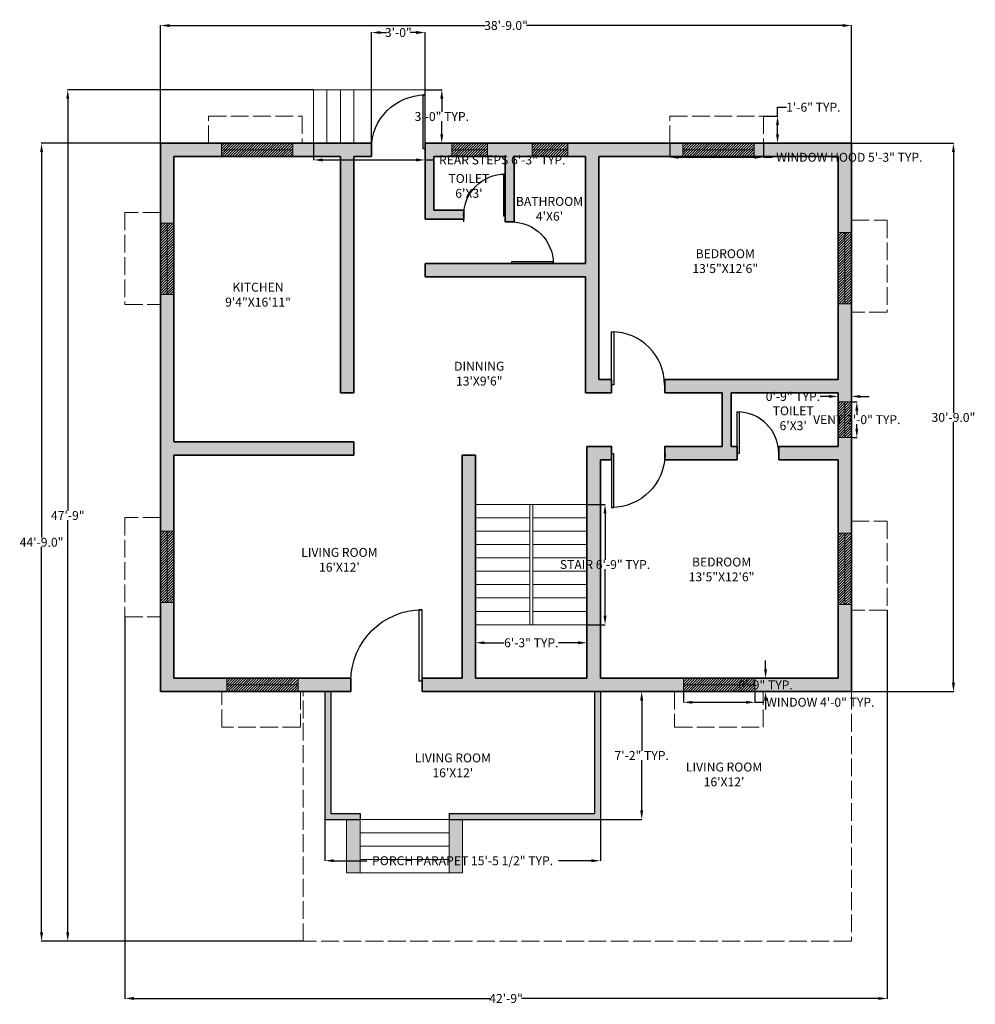
# Model space of a CAD drawing. Units: inches. Extents: x 1966 to 4198, y 2607 to 3884.
# Tile 2 of 8: x 1966 to 2609, y 3221 to 3884. Entities that reach past the tile are written whole.
import ezdxf

# ---------------------------------------------------------------- set-up
doc = ezdxf.new("R2010")
doc.units = ezdxf.units.IN
doc.header["$MEASUREMENT"] = 0
doc.linetypes.add('ACAD_ISO02W100', pattern=[15, 12, -3])
for name, color, linetype, lineweight in [('A-AREA-IDEN', 1, 'Continuous', 18), ('A-FLOR', 7, 'Continuous', 25), ('A-FLOR-PATT', 9, 'Continuous', 13), ('A-FLOR-STRS', 7, 'Continuous', 18), ('A-GLAZ', 4, 'Continuous', 18), ('A-GLAZ-PATT', 14, 'Continuous', 13), ('A-ROOF-OVHD', 17, 'ACAD_ISO02W100', 13), ('A-WALL', 7, 'Continuous', 35), ('A-WALL-PATT', 252, 'Continuous', 13), ('C-PRKG', 10, 'ACAD_ISO02W100', 18), ('dimension', 90, 'Continuous', 18), ('door', 17, 'Continuous', 25)]:
    doc.layers.add(name, color=color, linetype=linetype, lineweight=lineweight)
doc.styles.get("Standard").update_dxf_attribs({"font": 'arial.ttf'})
doc.dimstyles.get("Standard").update_dxf_attribs({"dimtxt": 6, "dimasz": 6, "dimexe": 0.18, "dimexo": 0.0625, "dimgap": 0.09, "dimtad": 0, "dimtih": 1, "dimtoh": 1, "dimdec": 1, "dimzin": 0, "dimdsep": 46, "dimlunit": 3, "dimtxsty": 'Standard', "dimcen": 0.09, "dimadec": 0, "dimazin": 0, "dimtfac": 1, "dimtdec": 1, "dimtofl": 0, "dimtmove": 0, "dimatfit": 3, "dimfxl": 1, "dimtolj": 1, "dimtzin": 0, "dimarcsym": 0})

# ---------------------------------------------------------------- blocks, each defined once
blk = doc.blocks.new('*U2')
for p, q in [((0, 0), (0, -6)), ((40, 0), (40, -6))]:
    blk.add_line(p, q)
blk.add_lwpolyline([(0, 0), (0, 40), (1.75, 40), (1.75, 0)], close=True)
blk.add_arc((0, 0), 40, 0, 90)
blk = doc.blocks.new('*D3')
at = {"layer": 'Defpoints', "color": 0, "transparency": 16777216}
for p in [(2060.47, 3800.5), (1980.34, 3263.5), (2156.44, 3263.5)]:
    blk.add_point(p, dxfattribs=at)
at = {"layer": 'dimension', "color": 0, "lineweight": -2, "transparency": 16777216}
for p, q in [((2060.41, 3800.5), (1980.16, 3800.5)), ((1980.34, 3794.5), (1980.34, 3535.16)), ((1980.34, 3269.5), (1980.34, 3528.85)), ((2156.37, 3263.5), (1980.16, 3263.5))]:
    blk.add_line(p, q, dxfattribs=at)
at = {"layer": 'dimension', "color": 0, "transparency": 16777216}
for points in [[(1979.34, 3794.5), (1981.34, 3794.5), (1980.34, 3800.5)], [(1979.34, 3269.5), (1981.34, 3269.5), (1980.34, 3263.5)]]:
    blk.add_solid(points, dxfattribs=at)
at = {"layer": 'dimension', "color": 0, "transparency": 16777216, "insert": (1980.34, 3532), "char_height": 6, "attachment_point": 5}
blk.add_mtext('\\A1;44\'-9.0"', dxfattribs=at)
blk = doc.blocks.new('*D4')
at = {"layer": 'Defpoints', "color": 0, "transparency": 16777216}
for p in [(2525.47, 3879.7), (2060.47, 3800.5), (2525.47, 3800.5)]:
    blk.add_point(p, dxfattribs=at)
at = {"layer": 'dimension', "color": 0, "lineweight": -2, "transparency": 16777216}
for p, q in [((2060.47, 3800.57), (2060.47, 3879.88)), ((2066.47, 3879.7), (2279.09, 3879.7)), ((2519.47, 3879.7), (2306.86, 3879.7)), ((2525.47, 3800.57), (2525.47, 3879.88))]:
    blk.add_line(p, q, dxfattribs=at)
at = {"layer": 'dimension', "color": 0, "transparency": 16777216}
for points in [[(2066.47, 3880.7), (2066.47, 3878.7), (2060.47, 3879.7)], [(2519.47, 3880.7), (2519.47, 3878.7), (2525.47, 3879.7)]]:
    blk.add_solid(points, dxfattribs=at)
at = {"layer": 'dimension', "color": 0, "transparency": 16777216, "insert": (2292.97, 3879.7), "char_height": 6, "attachment_point": 5}
blk.add_mtext('\\A1;38\'-9.0"', dxfattribs=at)
blk = doc.blocks.new('*D5')
at = {"layer": 'Defpoints', "color": 0, "transparency": 16777216}
for p in [(2525.47, 3800.5), (2525.47, 3431.5), (2594.13, 3431.5)]:
    blk.add_point(p, dxfattribs=at)
at = {"layer": 'dimension', "color": 0, "lineweight": -2, "transparency": 16777216}
for p, q in [((2525.54, 3800.5), (2594.31, 3800.5)), ((2594.13, 3794.5), (2594.13, 3619.16)), ((2594.13, 3437.5), (2594.13, 3612.85)), ((2525.54, 3431.5), (2594.31, 3431.5))]:
    blk.add_line(p, q, dxfattribs=at)
at = {"layer": 'dimension', "color": 0, "transparency": 16777216}
for points in [[(2593.13, 3794.5), (2595.13, 3794.5), (2594.13, 3800.5)], [(2593.13, 3437.5), (2595.13, 3437.5), (2594.13, 3431.5)]]:
    blk.add_solid(points, dxfattribs=at)
at = {"layer": 'dimension', "color": 0, "transparency": 16777216, "insert": (2594.13, 3616), "char_height": 6, "attachment_point": 5}
blk.add_mtext('\\A1;30\'-9.0"', dxfattribs=at)
blk = doc.blocks.new('WIN-48-PLAN')
for p, q in [((0, 9), (0, 0)), ((48, 9), (48, 0)), ((0, 4.5), (48, 4.5))]:
    blk.add_line(p, q)
blk = doc.blocks.new('VENT-24-PLAN')
for p, q in [((0, 0), (0, 9)), ((24, 0), (24, 9)), ((0, 4.5), (24, 4.5))]:
    blk.add_line(p, q)
blk = doc.blocks.new('STAIR-DOGLEG-PLAN')
for p, q in [((0, 81), (75, 81)), ((36.5, 0), (36.5, 81)), ((38.5, 0), (38.5, 81)), ((0, 72), (36.5, 72)), ((38.5, 72), (75, 72)), ((0, 63), (36.5, 63)), ((38.5, 63), (75, 63)), ((0, 54), (36.5, 54)), ((38.5, 54), (75, 54)), ((0, 45), (36.5, 45)), ((38.5, 45), (75, 45)), ((0, 36), (36.5, 36)), ((38.5, 36), (75, 36)), ((0, 27), (36.5, 27)), ((38.5, 27), (75, 27)), ((0, 18), (36.5, 18)), ((38.5, 18), (75, 18)), ((0, 9), (36.5, 9)), ((38.5, 9), (75, 9)), ((0, 0), (75, 0))]:
    blk.add_line(p, q)
blk = doc.blocks.new('REAR-ENTRY-STEPS')
for p, q in [((0, 36), (0, 0)), ((0, 36), (27, 36)), ((9, 36), (9, 0)), ((18, 36), (18, 0)), ((75, 36), (27, 36)), ((27, 36), (27, 0)), ((75, 0), (75, 36))]:
    blk.add_line(p, q)
blk = doc.blocks.new('PORCH-ENTRY-STEPS')
for p, q in [((0, 36), (0, 0)), ((9, 36), (9, 0)), ((9, 36), (69, 36)), ((69, 0), (69, 36)), ((78, 0), (78, 36)), ((9, 27), (69, 27)), ((9, 18), (69, 18)), ((9, 9), (69, 9)), ((9, 0), (0, 0)), ((9, 0), (69, 0)), ((69, 0), (78, 0))]:
    blk.add_line(p, q)
blk = doc.blocks.new('PORCH-PARAPET-PLAN')
for p, q in [((0, 86), (0, 0)), ((4, 86), (4, 4)), ((181.42, 86), (181.42, 4)), ((185.42, 86), (185.42, 0)), ((0, 0), (23.64, 0)), ((4, 4), (23.64, 4)), ((23.64, 4), (23.64, 0)), ((83.64, 4), (83.64, 0)), ((83.64, 4), (181.42, 4)), ((83.64, 0), (185.42, 0))]:
    blk.add_line(p, q)
blk = doc.blocks.new('WINDOW-HOOD-PLAN')
for p, q in [((0, 0), (0, 18.23)), ((0, 18.23), (63.03, 18.23)), ((63.03, 18.23), (63.03, 0))]:
    blk.add_line(p, q)
blk = doc.blocks.new('*D43')
at = {"layer": 'Defpoints', "color": 0, "transparency": 16777216}
for p in [(2412.47, 3431.5), (2460.47, 3431.5), (2460.47, 3424.3)]:
    blk.add_point(p, dxfattribs=at)
at = {"layer": 'dimension', "color": 0, "lineweight": -2, "transparency": 16777216}
for p, q in [((2412.47, 3431.44), (2412.47, 3424.12)), ((2460.47, 3431.44), (2460.47, 3424.12)), ((2418.47, 3424.3), (2454.47, 3424.3)), ((2460.47, 3424.3), (2466.47, 3424.3))]:
    blk.add_line(p, q, dxfattribs=at)
at = {"layer": 'dimension', "color": 0, "transparency": 16777216}
for points in [[(2418.47, 3425.3), (2418.47, 3423.3), (2412.47, 3424.3)], [(2454.47, 3425.3), (2454.47, 3423.3), (2460.47, 3424.3)]]:
    blk.add_solid(points, dxfattribs=at)
at = {"layer": 'dimension', "color": 0, "transparency": 16777216, "insert": (2504.53, 3424.3), "char_height": 6, "attachment_point": 5}
blk.add_mtext('\\A1;WINDOW 4\'-0" TYP.', dxfattribs=at)
blk = doc.blocks.new('*D44')
at = {"layer": 'Defpoints', "color": 0, "transparency": 16777216}
for p in [(2460.47, 3440.5), (2467.67, 3440.5), (2460.47, 3431.5)]:
    blk.add_point(p, dxfattribs=at)
at = {"layer": 'dimension', "color": 0, "lineweight": -2, "transparency": 16777216}
for p, q in [((2467.67, 3446.5), (2467.67, 3452.5)), ((2460.54, 3440.5), (2467.85, 3440.5)), ((2460.54, 3431.5), (2467.85, 3431.5)), ((2467.67, 3425.5), (2467.67, 3419.5))]:
    blk.add_line(p, q, dxfattribs=at)
at = {"layer": 'dimension', "color": 0, "transparency": 16777216}
for points in [[(2466.67, 3446.5), (2468.67, 3446.5), (2467.67, 3440.5)], [(2466.67, 3425.5), (2468.67, 3425.5), (2467.67, 3431.5)]]:
    blk.add_solid(points, dxfattribs=at)
at = {"layer": 'dimension', "color": 0, "transparency": 16777216, "insert": (2467.67, 3436), "char_height": 6, "attachment_point": 5}
blk.add_mtext('\\A1;0\'-9" TYP.', dxfattribs=at)
blk = doc.blocks.new('*D49')
at = {"layer": 'Defpoints', "color": 0, "transparency": 16777216}
for p in [(2525.47, 3626.5), (2529.07, 3626.5), (2525.47, 3602.5)]:
    blk.add_point(p, dxfattribs=at)
at = {"layer": 'dimension', "color": 0, "lineweight": -2, "transparency": 16777216}
for p, q in [((2525.54, 3626.5), (2529.25, 3626.5)), ((2529.07, 3620.5), (2529.07, 3617.66)), ((2529.07, 3608.5), (2529.07, 3611.35)), ((2525.54, 3602.5), (2529.25, 3602.5))]:
    blk.add_line(p, q, dxfattribs=at)
at = {"layer": 'dimension', "color": 0, "transparency": 16777216}
for points in [[(2528.07, 3620.5), (2530.07, 3620.5), (2529.07, 3626.5)], [(2528.07, 3608.5), (2530.07, 3608.5), (2529.07, 3602.5)]]:
    blk.add_solid(points, dxfattribs=at)
at = {"layer": 'dimension', "color": 0, "transparency": 16777216, "insert": (2529.07, 3614.5), "char_height": 6, "attachment_point": 5}
blk.add_mtext('\\A1;VENT 2\'-0" TYP.', dxfattribs=at)
blk = doc.blocks.new('*D50')
at = {"layer": 'Defpoints', "color": 0, "transparency": 16777216}
for p in [(2516.47, 3630.1), (2516.47, 3626.5), (2525.47, 3626.5)]:
    blk.add_point(p, dxfattribs=at)
at = {"layer": 'dimension', "color": 0, "lineweight": -2, "transparency": 16777216}
for p, q in [((2510.47, 3630.1), (2504.47, 3630.1)), ((2516.47, 3626.57), (2516.47, 3630.28)), ((2525.47, 3626.57), (2525.47, 3630.28)), ((2531.47, 3630.1), (2537.47, 3630.1))]:
    blk.add_line(p, q, dxfattribs=at)
at = {"layer": 'dimension', "color": 0, "transparency": 16777216}
for points in [[(2510.47, 3631.1), (2510.47, 3629.1), (2516.47, 3630.1)], [(2531.47, 3631.1), (2531.47, 3629.1), (2525.47, 3630.1)]]:
    blk.add_solid(points, dxfattribs=at)
at = {"layer": 'dimension', "color": 0, "transparency": 16777216, "insert": (2486.1, 3630.1), "char_height": 6, "attachment_point": 5}
blk.add_mtext('\\A1;0\'-9" TYP.', dxfattribs=at)
blk = doc.blocks.new('*D53')
at = {"layer": 'Defpoints', "color": 0, "transparency": 16777216}
for p in [(2347.47, 3557.5), (2359.62, 3557.5), (2347.47, 3476.5)]:
    blk.add_point(p, dxfattribs=at)
at = {"layer": 'dimension', "color": 0, "lineweight": -2, "transparency": 16777216}
for p, q in [((2347.54, 3557.5), (2359.8, 3557.5)), ((2359.62, 3551.5), (2359.62, 3520.2)), ((2359.62, 3482.5), (2359.62, 3513.81)), ((2347.54, 3476.5), (2359.8, 3476.5))]:
    blk.add_line(p, q, dxfattribs=at)
at = {"layer": 'dimension', "color": 0, "transparency": 16777216}
for points in [[(2358.62, 3551.5), (2360.62, 3551.5), (2359.62, 3557.5)], [(2358.62, 3482.5), (2360.62, 3482.5), (2359.62, 3476.5)]]:
    blk.add_solid(points, dxfattribs=at)
at = {"layer": 'dimension', "color": 0, "transparency": 16777216, "insert": (2359.62, 3517), "char_height": 6, "attachment_point": 5}
blk.add_mtext('\\A1;STAIR 6\'-9" TYP.', dxfattribs=at)
blk = doc.blocks.new('*D54')
at = {"layer": 'Defpoints', "color": 0, "transparency": 16777216}
for p in [(2272.47, 3476.5), (2347.47, 3476.5), (2347.47, 3464.35)]:
    blk.add_point(p, dxfattribs=at)
at = {"layer": 'dimension', "color": 0, "lineweight": -2, "transparency": 16777216}
for p, q in [((2272.47, 3476.44), (2272.47, 3464.17)), ((2347.47, 3476.44), (2347.47, 3464.17)), ((2278.47, 3464.35), (2291.58, 3464.35)), ((2341.47, 3464.35), (2328.37, 3464.35))]:
    blk.add_line(p, q, dxfattribs=at)
at = {"layer": 'dimension', "color": 0, "transparency": 16777216}
for points in [[(2278.47, 3465.35), (2278.47, 3463.35), (2272.47, 3464.35)], [(2341.47, 3465.35), (2341.47, 3463.35), (2347.47, 3464.35)]]:
    blk.add_solid(points, dxfattribs=at)
at = {"layer": 'dimension', "color": 0, "transparency": 16777216, "insert": (2309.97, 3464.35), "char_height": 6, "attachment_point": 5}
blk.add_mtext('\\A1;6\'-3" TYP.', dxfattribs=at)
blk = doc.blocks.new('*D55')
at = {"layer": 'Defpoints', "color": 0, "transparency": 16777216}
for p in [(2163.47, 3800.5), (2238.47, 3800.5), (2238.47, 3789.25)]:
    blk.add_point(p, dxfattribs=at)
at = {"layer": 'dimension', "color": 0, "lineweight": -2, "transparency": 16777216}
for p, q in [((2163.47, 3800.44), (2163.47, 3789.07)), ((2238.47, 3800.44), (2238.47, 3789.07)), ((2169.47, 3789.25), (2232.47, 3789.25)), ((2238.47, 3789.25), (2244.47, 3789.25))]:
    blk.add_line(p, q, dxfattribs=at)
at = {"layer": 'dimension', "color": 0, "transparency": 16777216}
for points in [[(2169.47, 3790.25), (2169.47, 3788.25), (2163.47, 3789.25)], [(2232.47, 3790.25), (2232.47, 3788.25), (2238.47, 3789.25)]]:
    blk.add_solid(points, dxfattribs=at)
at = {"layer": 'dimension', "color": 0, "transparency": 16777216, "insert": (2290.41, 3789.25), "char_height": 6, "attachment_point": 5}
blk.add_mtext('\\A1;REAR STEPS 6\'-3" TYP.', dxfattribs=at)
blk = doc.blocks.new('*D56')
at = {"layer": 'Defpoints', "color": 0, "transparency": 16777216}
for p in [(2238.47, 3836.5), (2249.72, 3836.5), (2238.47, 3800.5)]:
    blk.add_point(p, dxfattribs=at)
at = {"layer": 'dimension', "color": 0, "lineweight": -2, "transparency": 16777216}
for p, q in [((2238.54, 3836.5), (2249.9, 3836.5)), ((2249.72, 3830.5), (2249.72, 3821.66)), ((2249.72, 3806.5), (2249.72, 3815.35)), ((2238.54, 3800.5), (2249.9, 3800.5))]:
    blk.add_line(p, q, dxfattribs=at)
at = {"layer": 'dimension', "color": 0, "transparency": 16777216}
for points in [[(2248.72, 3830.5), (2250.72, 3830.5), (2249.72, 3836.5)], [(2248.72, 3806.5), (2250.72, 3806.5), (2249.72, 3800.5)]]:
    blk.add_solid(points, dxfattribs=at)
at = {"layer": 'dimension', "color": 0, "transparency": 16777216, "insert": (2249.72, 3818.5), "char_height": 6, "attachment_point": 5}
blk.add_mtext('\\A1;3\'-0" TYP.', dxfattribs=at)
blk = doc.blocks.new('*D59')
at = {"layer": 'Defpoints', "color": 0, "transparency": 16777216}
for p in [(2171.06, 3345.5), (2356.47, 3345.5), (2356.47, 3317.69)]:
    blk.add_point(p, dxfattribs=at)
at = {"layer": 'dimension', "color": 0, "lineweight": -2, "transparency": 16777216}
for p, q in [((2171.06, 3345.44), (2171.06, 3317.51)), ((2356.47, 3345.44), (2356.47, 3317.51)), ((2177.06, 3317.69), (2199.19, 3317.69)), ((2350.47, 3317.69), (2328.34, 3317.69))]:
    blk.add_line(p, q, dxfattribs=at)
at = {"layer": 'dimension', "color": 0, "transparency": 16777216}
for points in [[(2177.06, 3318.69), (2177.06, 3316.69), (2171.06, 3317.69)], [(2350.47, 3318.69), (2350.47, 3316.69), (2356.47, 3317.69)]]:
    blk.add_solid(points, dxfattribs=at)
at = {"layer": 'dimension', "color": 0, "transparency": 16777216, "insert": (2263.77, 3317.69), "char_height": 6, "attachment_point": 5}
blk.add_mtext('\\A1;PORCH PARAPET 15\'-5 1/2" TYP.', dxfattribs=at)
blk = doc.blocks.new('*D60')
at = {"layer": 'Defpoints', "color": 0, "transparency": 16777216}
for p in [(2356.47, 3431.5), (2384.29, 3431.5), (2356.47, 3345.5)]:
    blk.add_point(p, dxfattribs=at)
at = {"layer": 'dimension', "color": 0, "lineweight": -2, "transparency": 16777216}
for p, q in [((2356.54, 3431.5), (2384.47, 3431.5)), ((2384.29, 3425.5), (2384.29, 3391.61)), ((2384.29, 3351.5), (2384.29, 3385.4)), ((2356.54, 3345.5), (2384.47, 3345.5))]:
    blk.add_line(p, q, dxfattribs=at)
at = {"layer": 'dimension', "color": 0, "transparency": 16777216}
for points in [[(2383.29, 3425.5), (2385.29, 3425.5), (2384.29, 3431.5)], [(2383.29, 3351.5), (2385.29, 3351.5), (2384.29, 3345.5)]]:
    blk.add_solid(points, dxfattribs=at)
at = {"layer": 'dimension', "color": 0, "transparency": 16777216, "insert": (2384.29, 3388.5), "char_height": 6, "attachment_point": 5}
blk.add_mtext('\\A1;7\'-2" TYP.', dxfattribs=at)
blk = doc.blocks.new('*D61')
at = {"layer": 'Defpoints', "color": 0, "transparency": 16777216}
for p in [(2403.23, 3800.5), (2466.27, 3800.5), (2466.27, 3791.05)]:
    blk.add_point(p, dxfattribs=at)
at = {"layer": 'dimension', "color": 0, "lineweight": -2, "transparency": 16777216}
for p, q in [((2403.23, 3800.44), (2403.23, 3790.87)), ((2466.27, 3800.44), (2466.27, 3790.87)), ((2409.23, 3791.05), (2460.27, 3791.05)), ((2466.27, 3791.05), (2472.27, 3791.05))]:
    blk.add_line(p, q, dxfattribs=at)
at = {"layer": 'dimension', "color": 0, "transparency": 16777216}
for points in [[(2409.23, 3792.05), (2409.23, 3790.05), (2403.23, 3791.05)], [(2460.27, 3792.05), (2460.27, 3790.05), (2466.27, 3791.05)]]:
    blk.add_solid(points, dxfattribs=at)
at = {"layer": 'dimension', "color": 0, "transparency": 16777216, "insert": (2524.06, 3791.05), "char_height": 6, "attachment_point": 5}
blk.add_mtext('\\A1;WINDOW HOOD 5\'-3" TYP.', dxfattribs=at)
blk = doc.blocks.new('*D62')
at = {"layer": 'Defpoints', "color": 0, "transparency": 16777216}
for p in [(2466.27, 3818.73), (2475.72, 3818.73), (2466.27, 3800.5)]:
    blk.add_point(p, dxfattribs=at)
at = {"layer": 'dimension', "color": 0, "lineweight": -2, "transparency": 16777216}
for p, q in [((2475.72, 3818.73), (2475.72, 3824.73)), ((2475.72, 3824.73), (2481.72, 3824.73)), ((2466.33, 3818.73), (2475.9, 3818.73)), ((2475.72, 3806.5), (2475.72, 3812.73)), ((2466.33, 3800.5), (2475.9, 3800.5))]:
    blk.add_line(p, q, dxfattribs=at)
at = {"layer": 'dimension', "color": 0, "transparency": 16777216}
for points in [[(2474.72, 3812.73), (2476.72, 3812.73), (2475.72, 3818.73)], [(2474.72, 3806.5), (2476.72, 3806.5), (2475.72, 3800.5)]]:
    blk.add_solid(points, dxfattribs=at)
at = {"layer": 'dimension', "color": 0, "transparency": 16777216, "insert": (2499.82, 3824.73), "char_height": 6, "attachment_point": 5}
blk.add_mtext('\\A1;1\'-6" TYP.', dxfattribs=at)
blk = doc.blocks.new('*D83')
at = {"layer": 'Defpoints', "color": 0, "transparency": 16777216}
for p in [(2549.47, 3486.31), (2036.47, 3481.8), (2549.47, 3225)]:
    blk.add_point(p, dxfattribs=at)
at = {"layer": 'dimension', "color": 0, "lineweight": -2, "transparency": 16777216}
for p, q in [((2549.47, 3486.24), (2549.47, 3224.82)), ((2036.47, 3481.73), (2036.47, 3224.82)), ((2042.47, 3225), (2282.46, 3225)), ((2543.47, 3225), (2303.49, 3225))]:
    blk.add_line(p, q, dxfattribs=at)
at = {"layer": 'dimension', "color": 0, "transparency": 16777216}
for points in [[(2042.47, 3226), (2042.47, 3224), (2036.47, 3225)], [(2543.47, 3226), (2543.47, 3224), (2549.47, 3225)]]:
    blk.add_solid(points, dxfattribs=at)
at = {"layer": 'dimension', "color": 0, "transparency": 16777216, "insert": (2292.97, 3225), "char_height": 6, "attachment_point": 5}
blk.add_mtext('\\A1;42\'-9"', dxfattribs=at)
blk = doc.blocks.new('*D84')
at = {"layer": 'Defpoints', "color": 0, "transparency": 16777216}
for p in [(2163.47, 3836.5), (1997.97, 3263.5), (2156.44, 3263.5)]:
    blk.add_point(p, dxfattribs=at)
at = {"layer": 'dimension', "color": 0, "lineweight": -2, "transparency": 16777216}
for p, q in [((2163.41, 3836.5), (1997.79, 3836.5)), ((1997.97, 3830.5), (1997.97, 3553.16)), ((1997.97, 3269.5), (1997.97, 3546.85)), ((2156.37, 3263.5), (1997.79, 3263.5))]:
    blk.add_line(p, q, dxfattribs=at)
at = {"layer": 'dimension', "color": 0, "transparency": 16777216}
for points in [[(1996.97, 3830.5), (1998.97, 3830.5), (1997.97, 3836.5)], [(1996.97, 3269.5), (1998.97, 3269.5), (1997.97, 3263.5)]]:
    blk.add_solid(points, dxfattribs=at)
at = {"layer": 'dimension', "color": 0, "transparency": 16777216, "insert": (1997.97, 3550), "char_height": 6, "attachment_point": 5}
blk.add_mtext('\\A1;47\'-9"', dxfattribs=at)
blk = doc.blocks.new('*D86')
at = {"layer": 'Defpoints', "color": 0, "transparency": 16777216}
for p in [(2238.47, 3875), (2202.47, 3800.5), (2238.47, 3800.5)]:
    blk.add_point(p, dxfattribs=at)
at = {"layer": 'dimension', "color": 0, "lineweight": -2, "transparency": 16777216}
for p, q in [((2202.47, 3800.57), (2202.47, 3875.18)), ((2208.47, 3875), (2212.41, 3875)), ((2232.47, 3875), (2228.54, 3875)), ((2238.47, 3800.57), (2238.47, 3875.18))]:
    blk.add_line(p, q, dxfattribs=at)
at = {"layer": 'dimension', "color": 0, "transparency": 16777216}
for points in [[(2208.47, 3876), (2208.47, 3874), (2202.47, 3875)], [(2232.47, 3876), (2232.47, 3874), (2238.47, 3875)]]:
    blk.add_solid(points, dxfattribs=at)
at = {"layer": 'dimension', "color": 0, "transparency": 16777216, "insert": (2220.47, 3875), "char_height": 6, "attachment_point": 5}
blk.add_mtext('\\A1;3\'-0"', dxfattribs=at)

msp = doc.modelspace()

# ---------------------------------------------------------------- hatches: boundary and pattern name
at = {"layer": 'A-FLOR-PATT'}
h = msp.add_hatch(color=256, dxfattribs=at)
h.dxf.hatch_style = 1
h.paths.add_polyline_path([(2194.7, 3345.5), (2185.7, 3345.5), (2185.7, 3309.5), (2194.7, 3309.5)])
h.paths.add_polyline_path([(2263.7, 3345.5), (2254.7, 3345.5), (2254.7, 3309.5), (2263.7, 3309.5)])
at = {"layer": 'A-GLAZ-PATT'}
h = msp.add_hatch(dxfattribs=at)
h.set_pattern_fill('ANSI31', color=256, scale=10)
h.paths.add_polyline_path([(2064.97, 3746.62), (2060.47, 3746.62), (2060.47, 3698.62), (2064.97, 3698.62)])
h.paths.add_polyline_path([(2069.47, 3746.62), (2064.97, 3746.62), (2064.97, 3698.62), (2069.47, 3698.62)])
h.paths.add_polyline_path([(2149.47, 3800.5), (2101.47, 3800.5), (2101.47, 3796), (2149.47, 3796)])
h.paths.add_polyline_path([(2149.47, 3796), (2101.47, 3796), (2101.47, 3791.5), (2149.47, 3791.5)])
h.paths.add_polyline_path([(2280.47, 3800.5), (2256.47, 3800.5), (2256.47, 3796), (2280.47, 3796)])
h.paths.add_polyline_path([(2280.47, 3796), (2256.47, 3796), (2256.47, 3791.5), (2280.47, 3791.5)])
h.paths.add_polyline_path([(2334.47, 3800.5), (2310.47, 3800.5), (2310.47, 3796), (2334.47, 3796)])
h.paths.add_polyline_path([(2334.47, 3796), (2310.47, 3796), (2310.47, 3791.5), (2334.47, 3791.5)])
h.paths.add_polyline_path([(2459.97, 3800.5), (2411.97, 3800.5), (2411.97, 3796), (2459.97, 3796)])
h.paths.add_polyline_path([(2459.97, 3796), (2411.97, 3796), (2411.97, 3791.5), (2459.97, 3791.5)])
h.paths.add_polyline_path([(2525.47, 3740.5), (2520.97, 3740.5), (2520.97, 3692.5), (2525.47, 3692.5)])
h.paths.add_polyline_path([(2520.97, 3740.5), (2516.47, 3740.5), (2516.47, 3692.5), (2520.97, 3692.5)])
h.paths.add_polyline_path([(2520.97, 3626.5), (2516.47, 3626.5), (2516.47, 3602.5), (2520.97, 3602.5)])
h.paths.add_polyline_path([(2525.47, 3626.5), (2520.97, 3626.5), (2520.97, 3602.5), (2525.47, 3602.5)])
h.paths.add_polyline_path([(2525.47, 3538), (2520.97, 3538), (2520.97, 3490), (2525.47, 3490)])
h.paths.add_polyline_path([(2520.97, 3538), (2516.47, 3538), (2516.47, 3490), (2520.97, 3490)])
h.paths.add_polyline_path([(2460.47, 3436), (2412.47, 3436), (2412.47, 3431.5), (2460.47, 3431.5)])
h.paths.add_polyline_path([(2460.47, 3440.5), (2412.47, 3440.5), (2412.47, 3436), (2460.47, 3436)])
h = msp.add_hatch(dxfattribs=at)
h.set_pattern_fill('ANSI31', color=256, scale=10)
h.paths.add_polyline_path([(2152.97, 3440.5), (2104.97, 3440.5), (2104.97, 3436), (2152.97, 3436)])
h.paths.add_polyline_path([(2152.97, 3436), (2104.97, 3436), (2104.97, 3431.5), (2152.97, 3431.5)])
h.paths.add_polyline_path([(2064.97, 3539.5), (2060.47, 3539.5), (2060.47, 3491.5), (2064.97, 3491.5)])
h.paths.add_polyline_path([(2069.47, 3539.5), (2064.97, 3539.5), (2064.97, 3491.5), (2069.47, 3491.5)])
at = {"layer": 'A-WALL-PATT'}
h = msp.add_hatch(color=256, dxfattribs=at)
h.dxf.hatch_style = 1
h.paths.add_polyline_path([(2190.47, 3599.5), (2069.47, 3599.5), (2069.47, 3698.62), (2060.47, 3698.62), (2060.47, 3590.5), (2060.47, 3539.5), (2069.47, 3539.5), (2069.47, 3590.5), (2190.47, 3590.5)])
h.paths.add_polyline_path([(2069.47, 3491.5), (2060.47, 3491.5), (2060.47, 3431.5), (2104.97, 3431.5), (2104.97, 3440.5), (2069.47, 3440.5)])
h.paths.add_polyline_path([(2188.46, 3440.5), (2152.97, 3440.5), (2152.97, 3431.5), (2188.46, 3431.5)])
h.paths.add_polyline_path([(2175.06, 3431.5), (2171.06, 3431.5), (2171.06, 3345.5), (2194.7, 3345.5), (2194.7, 3349.5), (2175.06, 3349.5)])
h.paths.add_polyline_path([(2412.47, 3440.5), (2356.47, 3440.5), (2356.47, 3587.5), (2363.95, 3587.5), (2363.95, 3591.41), (2363.95, 3596.5), (2347.47, 3596.5), (2347.47, 3440.5), (2272.47, 3440.5), (2272.47, 3590.5), (2263.47, 3590.5), (2263.47, 3440.5), (2236.46, 3440.5), (2236.46, 3438.68), (2236.46, 3431.5), (2272.47, 3431.5), (2412.47, 3431.5)])
h.paths.add_polyline_path([(2356.47, 3431.5), (2352.47, 3431.5), (2352.47, 3349.5), (2254.7, 3349.5), (2254.7, 3345.5), (2356.47, 3345.5)])
h.paths.add_polyline_path([(2525.47, 3490), (2516.47, 3490), (2516.47, 3440.5), (2460.47, 3440.5), (2460.47, 3431.5), (2525.47, 3431.5)])
h.paths.add_polyline_path([(2525.47, 3599.5), (2525.47, 3602.5), (2516.47, 3602.5), (2516.47, 3596.5), (2476.59, 3596.5), (2476.59, 3587.5), (2516.47, 3587.5), (2516.47, 3538), (2525.47, 3538)])
h.paths.add_polyline_path([(2444.47, 3632.5), (2516.47, 3632.5), (2516.47, 3626.5), (2525.47, 3626.5), (2525.47, 3692.5), (2516.47, 3692.5), (2516.47, 3641.5), (2399.95, 3641.5), (2399.95, 3632.5), (2438.47, 3632.5), (2438.47, 3596.5), (2399.99, 3596.5), (2399.99, 3591.41, -0.010779), (2399.95, 3589.86), (2399.95, 3587.5), (2448.59, 3587.5), (2448.59, 3591.7), (2448.59, 3596.5), (2444.47, 3596.5)])
h.paths.add_polyline_path([(2355.47, 3791.5), (2411.97, 3791.5), (2411.97, 3800.5), (2355.47, 3800.5), (2334.47, 3800.5), (2334.47, 3791.5), (2346.47, 3791.5), (2346.47, 3719.5), (2298.47, 3719.5), (2292.47, 3719.5), (2238.47, 3719.5), (2238.47, 3710.5), (2346.47, 3710.5), (2346.47, 3632.5), (2363.95, 3632.5), (2363.95, 3637.87), (2363.95, 3641.5), (2355.47, 3641.5)])
h.paths.add_polyline_path([(2525.47, 3800.5), (2459.97, 3800.5), (2459.97, 3791.5), (2516.47, 3791.5), (2516.47, 3740.5), (2525.47, 3740.5)])
h.paths.add_polyline_path([(2310.47, 3800.5), (2280.47, 3800.5), (2280.47, 3791.5), (2292.47, 3791.5), (2292.47, 3755.5), (2292.47, 3751.71), (2292.47, 3747.5), (2298.47, 3747.5), (2298.47, 3791.5), (2310.47, 3791.5)], flags=17)
h.paths.add_polyline_path([(2256.47, 3800.5), (2238.47, 3800.5), (2238.47, 3796.92), (2238.47, 3791.5), (2238.47, 3749.5), (2264.41, 3749.5), (2264.41, 3751.71, -0.016709), (2264.47, 3753.59), (2264.47, 3755.5), (2244.47, 3755.5), (2244.47, 3791.5), (2256.47, 3791.5)], flags=17)
h.paths.add_polyline_path([(2202.39, 3796.92, -0.017138), (2202.47, 3799.39), (2202.47, 3800.5), (2190.47, 3800.5), (2149.47, 3800.5), (2149.47, 3791.5), (2181.47, 3791.5), (2181.47, 3632.5), (2190.47, 3632.5), (2190.47, 3791.5), (2202.39, 3791.5)])
h.paths.add_polyline_path([(2101.47, 3800.5), (2060.47, 3800.5), (2060.47, 3746.62), (2069.47, 3746.62), (2069.47, 3791.5), (2101.47, 3791.5)])

# ---------------------------------------------------------------- linework, layer by layer
at = {"layer": 'A-GLAZ'}
msp.add_line((2516.47, 3538), (2525.47, 3538), dxfattribs=at)
msp.add_line((2516.47, 3538), (2525.47, 3538), dxfattribs=at)
at = {"layer": 'A-ROOF-OVHD'}
for p, q in [((2060.47, 3753.9), (2036.47, 3753.9)), ((2036.47, 3753.9), (2036.47, 3692.03)), ((2525.47, 3748.71), (2549.47, 3748.71)), ((2549.47, 3748.71), (2549.47, 3686.74)), ((2036.47, 3692.03), (2060.47, 3692.03)), ((2549.47, 3686.74), (2525.47, 3686.74)), ((2060.47, 3548.63), (2036.47, 3548.63)), ((2036.47, 3548.63), (2036.47, 3481.8)), ((2525.47, 3546.28), (2549.47, 3546.28)), ((2549.47, 3546.28), (2549.47, 3486.31)), ((2549.47, 3486.31), (2525.47, 3486.31)), ((2036.47, 3481.8), (2060.47, 3481.8)), ((2101.62, 3407.5), (2101.62, 3431.5)), ((2154.57, 3431.5), (2154.57, 3407.5)), ((2406.4, 3431.5), (2406.4, 3407.5)), ((2465.98, 3407.5), (2465.98, 3431.5)), ((2154.57, 3407.5), (2101.62, 3407.5)), ((2406.4, 3407.5), (2465.98, 3407.5))]:
    msp.add_line(p, q, dxfattribs=at)
at = {"layer": 'A-WALL'}
for p, q in [((2060.47, 3800.5), (2060.47, 3590.5)), ((2202.47, 3800.5), (2060.47, 3800.5)), ((2202.47, 3791.5), (2202.47, 3800.5)), ((2355.47, 3800.5), (2238.47, 3800.5)), ((2238.47, 3791.5), (2238.47, 3800.5)), ((2355.47, 3800.5), (2525.47, 3800.5)), ((2525.47, 3599.5), (2525.47, 3800.5)), ((2181.47, 3791.5), (2069.47, 3791.5)), ((2069.47, 3791.5), (2069.47, 3599.5)), ((2181.47, 3632.5), (2181.47, 3791.5)), ((2190.47, 3632.5), (2190.47, 3791.5)), ((2202.47, 3791.5), (2190.47, 3791.5)), ((2238.47, 3749.5), (2238.47, 3791.5)), ((2244.47, 3755.5), (2244.47, 3791.5)), ((2292.47, 3791.5), (2244.47, 3791.5)), ((2292.47, 3755.5), (2292.47, 3791.5)), ((2346.47, 3791.5), (2298.47, 3791.5)), ((2298.47, 3747.5), (2298.47, 3791.5)), ((2346.47, 3719.5), (2346.47, 3791.5)), ((2355.47, 3641.5), (2355.47, 3791.5)), ((2355.47, 3791.5), (2516.47, 3791.5)), ((2516.47, 3641.5), (2516.47, 3791.5)), ((2264.47, 3755.5), (2244.47, 3755.5)), ((2264.47, 3749.5), (2264.47, 3755.5)), ((2292.47, 3749.5), (2292.47, 3755.5)), ((2264.47, 3749.5), (2238.47, 3749.5)), ((2292.47, 3747.5), (2292.47, 3749.5)), ((2292.47, 3747.5), (2298.47, 3747.5)), ((2238.47, 3710.5), (2238.47, 3719.5)), ((2292.47, 3719.5), (2238.47, 3719.5)), ((2292.47, 3719.5), (2298.47, 3719.5)), ((2346.47, 3719.5), (2298.47, 3719.5)), ((2346.47, 3710.5), (2238.47, 3710.5)), ((2346.47, 3632.5), (2346.47, 3710.5)), ((2355.47, 3641.5), (2363.95, 3641.5)), ((2363.95, 3641.5), (2363.95, 3632.5)), ((2399.95, 3641.5), (2399.95, 3632.5)), ((2399.95, 3641.5), (2516.47, 3641.5)), ((2181.47, 3632.5), (2190.47, 3632.5)), ((2346.47, 3632.5), (2363.95, 3632.5)), ((2399.95, 3632.5), (2438.47, 3632.5)), ((2438.47, 3632.5), (2438.47, 3596.5)), ((2444.47, 3632.5), (2444.47, 3596.5)), ((2444.47, 3632.5), (2516.47, 3632.5)), ((2516.47, 3632.5), (2516.47, 3596.5)), ((2069.47, 3599.5), (2190.47, 3599.5)), ((2190.47, 3590.5), (2190.47, 3599.5)), ((2525.47, 3599.5), (2525.47, 3431.5)), ((2347.47, 3440.5), (2347.47, 3596.5)), ((2347.47, 3596.5), (2363.95, 3596.5)), ((2363.95, 3596.5), (2363.95, 3587.5)), ((2399.95, 3596.5), (2399.95, 3587.5)), ((2399.95, 3596.5), (2438.47, 3596.5)), ((2444.47, 3596.5), (2448.59, 3596.5)), ((2448.59, 3596.5), (2448.59, 3587.5)), ((2476.59, 3596.5), (2476.59, 3587.5)), ((2476.59, 3596.5), (2516.47, 3596.5)), ((2060.47, 3431.5), (2060.47, 3590.5)), ((2069.47, 3590.5), (2190.47, 3590.5)), ((2069.47, 3440.5), (2069.47, 3590.5)), ((2263.47, 3440.5), (2263.47, 3590.5)), ((2263.47, 3590.5), (2272.47, 3590.5)), ((2272.47, 3440.5), (2272.47, 3590.5)), ((2356.47, 3440.5), (2356.47, 3587.5)), ((2356.47, 3587.5), (2363.95, 3587.5)), ((2399.95, 3587.5), (2448.59, 3587.5)), ((2476.59, 3587.5), (2516.47, 3587.5)), ((2516.47, 3587.5), (2516.47, 3440.5)), ((2069.47, 3440.5), (2188.46, 3440.5)), ((2188.46, 3440.5), (2188.46, 3431.5)), ((2236.46, 3440.5), (2236.46, 3431.5)), ((2236.46, 3440.5), (2263.47, 3440.5)), ((2272.47, 3440.5), (2347.47, 3440.5)), ((2356.47, 3440.5), (2516.47, 3440.5)), ((2060.47, 3431.5), (2188.46, 3431.5)), ((2236.46, 3431.5), (2272.47, 3431.5)), ((2272.47, 3431.5), (2525.47, 3431.5))]:
    msp.add_line(p, q, dxfattribs=at)
at = {"layer": 'C-PRKG'}
for p, q in [((2156.44, 3263.5), (2156.44, 3431.5)), ((2525.47, 3431.5), (2525.47, 3263.5)), ((2525.47, 3263.5), (2156.44, 3263.5))]:
    msp.add_line(p, q, dxfattribs=at)

# ---------------------------------------------------------------- block references
at = {"layer": 'A-FLOR'}
msp.add_blockref('PORCH-PARAPET-PLAN', (2171.06, 3345.5), dxfattribs=at)
at = {"layer": 'A-FLOR-STRS'}
for name, p in [('REAR-ENTRY-STEPS', (2163.47, 3800.5)), ('STAIR-DOGLEG-PLAN', (2272.47, 3476.5)), ('PORCH-ENTRY-STEPS', (2185.7, 3309.5))]:
    msp.add_blockref(name, p, dxfattribs=at)
at = {"layer": 'A-GLAZ'}
for name, p, rotation in [('WIN-48-PLAN', (2149.47, 3800.5), 180), ('VENT-24-PLAN', (2334.47, 3800.5), 180), ('WIN-48-PLAN', (2459.97, 3800.5), 180), ('WIN-48-PLAN', (2060.47, 3746.62), 269.9999999999966), ('WIN-48-PLAN', (2516.47, 3740.5), 269.9999999999966), ('VENT-24-PLAN', (2525.48, 3602.5), 90.00000000000072), ('WIN-48-PLAN', (2060.47, 3539.5), 269.9999999999968), ('WIN-48-PLAN', (2516.47, 3538), 270.0000000000002), ('WIN-48-PLAN', (2152.97, 3440.5), 180)]:
    msp.add_blockref(name, p, dxfattribs=dict(at, rotation=rotation))
for name, p in [('VENT-24-PLAN', (2256.47, 3791.5)), ('WIN-48-PLAN', (2412.47, 3431.5))]:
    msp.add_blockref(name, p, dxfattribs=at)
at = {"layer": 'A-ROOF-OVHD'}
for p in [(2092.73, 3800.5), (2403.23, 3800.5)]:
    msp.add_blockref('WINDOW-HOOD-PLAN', p, dxfattribs=at)
at = {"layer": 'door'}
for p, xscale, yscale, zscale in [((2238.47, 3796.92), -0.902118520811191, 0.902118520811191, 0.902118520811191), ((2292.47, 3751.71), -0.7015660841111144, 0.7015660841111144, 0.7015660841111144), ((2363.95, 3637.87), 0.8937584040391099, 0.8937584040391099, 0.8937584040391099), ((2448.59, 3591.7), 0.699710970889911, 0.699710970889911, 0.699710970889911), ((2236.46, 3438.68), -1.196636277150106, 1.196636277150106, 1.196636277150106)]:
    msp.add_blockref('*U2', p, dxfattribs=dict(at, xscale=xscale, yscale=yscale, zscale=zscale))
for p, xscale, yscale, zscale, rotation in [((2296.68, 3719.5), -0.7015660841111144, 0.7015660841111144, 0.7015660841111144, 270), ((2363.95, 3591.41), -0.900837184831981, 0.900837184831981, 0.900837184831981, 180)]:
    msp.add_blockref('*U2', p, dxfattribs=dict(at, xscale=xscale, yscale=yscale, zscale=zscale, rotation=rotation))

# ---------------------------------------------------------------- texts
at = {"layer": 'A-AREA-IDEN', "char_height": 6, "attachment_point": 2}
for s, width, insert in [("TOILET\\P6'X3'", 45.6254, (2267.99, 3779.78)), ("BATHROOM\\P4'X6'", 45.6254, (2322.23, 3764.34)), ('BEDROOM\\P13\'5"X12\'6"', 45.6254, (2440.53, 3729.16)), ('KITCHEN\\P9\'4"X16\'11"', 45.6254, (2126.04, 3706.6)), ('DINNING\\P13\'X9\'6"', 45.6254, (2274.95, 3653.46)), ("TOILET\\P6'X3'", 45.6254, (2486.26, 3623.45)), ("LIVING ROOM\\P16'X12'", 89.9452, (2180.81, 3528.18)), ('BEDROOM\\P13\'5"X12\'6"', 45.6254, (2438.07, 3521.69)), ("LIVING ROOM\\P16'X12'", 89.9452, (2257.15, 3389.86)), ("LIVING ROOM\\P16'X12'", 89.9452, (2439.73, 3383.73))]:
    msp.add_mtext_dynamic_manual_height_columns(s, width=width, gutter_width=1, heights=[0], dxfattribs=dict(at, insert=insert))

# ---------------------------------------------------------------- dimensions: what is measured, and where the dimension line sits
at = {"layer": 'dimension'}
for base, p1, p2, override, picture, middle in [((2525.47, 3879.7), (2060.47, 3800.5), (2525.47, 3800.5), {"dimclrd": 0, "dimclre": 0, "dimclrt": 0}, '*D4', (2292.97, 3879.7)), ((2238.47, 3875), (2202.47, 3800.5), (2238.47, 3800.5), {"dimdec": 1, "dimlfac": 1, "dimrnd": 0, "dimzin": 1, "dimdsep": 46, "dimlunit": 4, "dimfrac": 2}, '*D86', (2220.47, 3875)), ((2549.47, 3225), (2036.47, 3481.8), (2549.47, 3486.31), {"dimdec": 1, "dimlfac": 1, "dimrnd": 0, "dimzin": 1, "dimdsep": 46, "dimlunit": 4, "dimfrac": 2}, '*D83', (2292.97, 3225))]:
    dim = msp.add_linear_dim(base=base, p1=p1, p2=p2, dimstyle='Standard', override=override, dxfattribs=at)
    dim.commit()
    dim.dimension.update_dxf_attribs({"geometry": picture, "text_midpoint": middle})
for base, p1, p2, override, picture, middle in [((1997.97, 3263.5), (2163.47, 3836.5), (2156.44, 3263.5), {"dimdec": 1, "dimlfac": 1, "dimrnd": 0, "dimzin": 1, "dimdsep": 46, "dimlunit": 4, "dimfrac": 2}, '*D84', (1997.97, 3550)), ((1980.34, 3263.5), (2060.47, 3800.5), (2156.44, 3263.5), {"dimclrd": 0, "dimclre": 0, "dimclrt": 0}, '*D3', (1980.34, 3532)), ((2594.13, 3431.5), (2525.47, 3800.5), (2525.47, 3431.5), {"dimclrd": 0, "dimclre": 0, "dimclrt": 0}, '*D5', (2594.13, 3616))]:
    dim = msp.add_linear_dim(base=base, p1=p1, p2=p2, angle=90, dimstyle='Standard', override=override, dxfattribs=at)
    dim.commit()
    dim.dimension.update_dxf_attribs({"geometry": picture, "text_midpoint": middle})
for base, p1, p2, angle, text, picture, middle in [((2249.72, 3836.5), (2238.47, 3800.5), (2238.47, 3836.5), 90, '<> TYP.', '*D56', (2249.72, 3818.5)), ((2475.72, 3818.73), (2466.27, 3800.5), (2466.27, 3818.73), 90, '<> TYP.', '*D62', (2499.82, 3824.73)), ((2516.47, 3630.1), (2525.47, 3626.5), (2516.47, 3626.5), 180, '<> TYP.', '*D50', (2486.1, 3630.1)), ((2529.07, 3626.5), (2525.47, 3602.5), (2525.47, 3626.5), 90, 'VENT <> TYP.', '*D49', (2529.07, 3614.5)), ((2359.62, 3557.5), (2347.47, 3476.5), (2347.47, 3557.5), 90, 'STAIR <> TYP.', '*D53', (2359.62, 3517)), ((2467.67, 3440.5), (2460.47, 3431.5), (2460.47, 3440.5), 90, '<> TYP.', '*D44', (2467.67, 3436)), ((2384.29, 3431.5), (2356.47, 3345.5), (2356.47, 3431.5), 90, '<> TYP.', '*D60', (2384.29, 3388.5))]:
    dim = msp.add_linear_dim(base=base, p1=p1, p2=p2, angle=angle, text=text, dimstyle='Standard', override={"dimdec": 1, "dimlfac": 1, "dimrnd": 0, "dimzin": 1, "dimdsep": 46, "dimlunit": 4, "dimfrac": 2}, dxfattribs=at)
    dim.commit()
    dim.dimension.update_dxf_attribs({"geometry": picture, "text_midpoint": middle})
for base, p1, p2, text, picture, middle in [((2466.27, 3791.05), (2403.23, 3800.5), (2466.27, 3800.5), 'WINDOW HOOD <> TYP.', '*D61', (2524.06, 3791.05)), ((2238.47, 3789.25), (2163.47, 3800.5), (2238.47, 3800.5), 'REAR STEPS <> TYP.', '*D55', (2290.41, 3789.25)), ((2347.47, 3464.35), (2272.47, 3476.5), (2347.47, 3476.5), '<> TYP.', '*D54', (2309.97, 3464.35)), ((2460.47, 3424.3), (2412.47, 3431.5), (2460.47, 3431.5), 'WINDOW <> TYP.', '*D43', (2504.53, 3424.3)), ((2356.47, 3317.69), (2171.06, 3345.5), (2356.47, 3345.5), 'PORCH PARAPET <> TYP.', '*D59', (2263.77, 3317.69))]:
    dim = msp.add_linear_dim(base=base, p1=p1, p2=p2, text=text, dimstyle='Standard', override={"dimdec": 1, "dimlfac": 1, "dimrnd": 0, "dimzin": 1, "dimdsep": 46, "dimlunit": 4, "dimfrac": 2}, dxfattribs=at)
    dim.commit()
    dim.dimension.update_dxf_attribs({"geometry": picture, "text_midpoint": middle})

doc.saveas('drawing.dxf')
